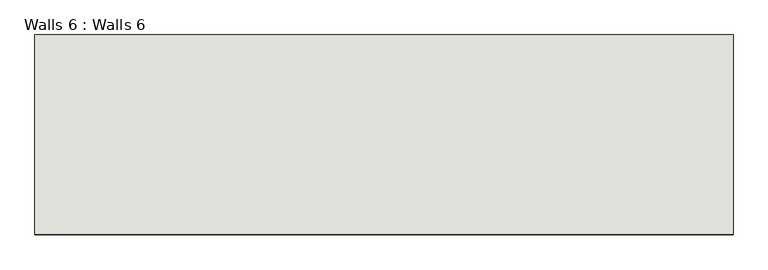
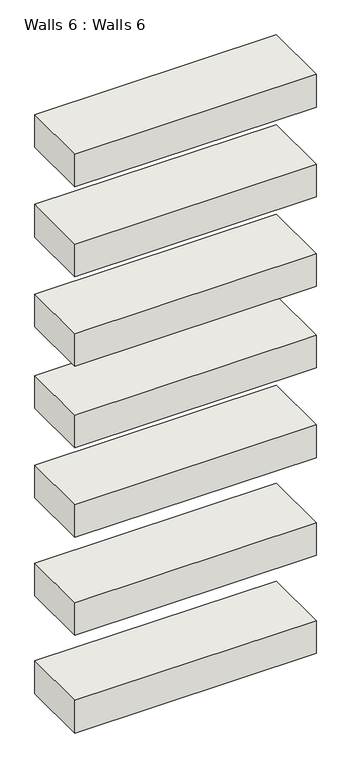
"""IFC4 building model written with IfcOpenShell, lengths in millimetres: wall geometry, Walls 6 : Walls 6."""

from ifc_helpers import new_model, si_unit, frame, origin, place, context, project, spatial, polyline, outline, extrude, source, transform, mapped, element, save


def walls_6_walls_6_ffd2a55d(model_context):
    return source(origin(), model_context, "Body", "SweptSolid", [
        extrude(outline(polyline([(-2720.1036351, 1505.9827135), (-3786.9036351, 1505.9827135), (-3786.9036351, 1810.7827135), (-2720.1036351, 1810.7827135), (-2720.1036351, 1505.9827135)])), frame((0.0, 0.0, 4076.7), z_axis=(0.0, 0.0, 1.0), x_axis=(1.0, 0.0, 0.0)), (0.0, 0.0, 1.0), 152.4),
        extrude(outline(polyline([(-2720.1036351, 1505.9827135), (-3786.9036351, 1505.9827135), (-3786.9036351, 1810.7827135), (-2720.1036351, 1810.7827135), (-2720.1036351, 1505.9827135)])), frame((0.0, 0.0, 3657.6), z_axis=(0.0, 0.0, 1.0), x_axis=(1.0, 0.0, 0.0)), (0.0, 0.0, 1.0), 152.4),
        extrude(outline(polyline([(-2720.1036351, 1505.9827135), (-3786.9036351, 1505.9827135), (-3786.9036351, 1810.7827135), (-2720.1036351, 1810.7827135), (-2720.1036351, 1505.9827135)])), frame((0.0, 0.0, 3238.5), z_axis=(0.0, 0.0, 1.0), x_axis=(1.0, 0.0, 0.0)), (0.0, 0.0, 1.0), 152.4),
        extrude(outline(polyline([(-2720.1036351, 1505.9827135), (-3786.9036351, 1505.9827135), (-3786.9036351, 1810.7827135), (-2720.1036351, 1810.7827135), (-2720.1036351, 1505.9827135)])), frame((0.0, 0.0, 2857.5), z_axis=(0.0, 0.0, 1.0), x_axis=(1.0, 0.0, 0.0)), (0.0, 0.0, 1.0), 152.4),
        extrude(outline(polyline([(-2720.1036351, 1505.9827135), (-3786.9036351, 1505.9827135), (-3786.9036351, 1810.7827135), (-2720.1036351, 1810.7827135), (-2720.1036351, 1505.9827135)])), frame((0.0, 0.0, 2438.4), z_axis=(0.0, 0.0, 1.0), x_axis=(1.0, 0.0, 0.0)), (0.0, 0.0, 1.0), 152.4),
        extrude(outline(polyline([(-2720.1036351, 1505.9827135), (-3786.9036351, 1505.9827135), (-3786.9036351, 1810.7827135), (-2720.1036351, 1810.7827135), (-2720.1036351, 1505.9827135)])), frame((0.0, 0.0, 1981.2), z_axis=(0.0, 0.0, 1.0), x_axis=(1.0, 0.0, 0.0)), (0.0, 0.0, 1.0), 152.4),
        extrude(outline(polyline([(-2720.1036351, 1505.9827135), (-3786.9036351, 1505.9827135), (-3786.9036351, 1810.7827135), (-2720.1036351, 1810.7827135), (-2720.1036351, 1505.9827135)])), frame((0.0, 0.0, 1524.0), z_axis=(0.0, 0.0, 1.0), x_axis=(1.0, 0.0, 0.0)), (0.0, 0.0, 1.0), 152.4),
    ])


if __name__ == "__main__":
    model = new_model("IFC4")
    model_context = context("Model", 3, world=origin())
    ifc_project = project(units=[si_unit("LENGTHUNIT", "METRE", prefix="MILLI")], contexts=[model_context])
    site = spatial("IfcSite", under=ifc_project)
    building = spatial("IfcBuilding", under=site)
    placement = place(None, origin())
    walls_6_walls_6_shape = walls_6_walls_6_ffd2a55d(model_context)
    element("IfcWall", 1, ObjectType="Walls 6 : Walls 6", at=placement, inside=building, context=model_context, shape_type="MappedRepresentation", body=[
        mapped(walls_6_walls_6_shape, transform((0.0, 0.0, 0.0), x_axis=(1.0, 0.0, 0.0), y_axis=(0.0, 1.0, 0.0), z_axis=(0.0, 0.0, 1.0))),
    ])
    save(model, "model.ifc")

# Revit data of these elements
# Element 1 (IfcWall, "Walls 6 : Walls 6")
#   Materials on its faces: "Default Wall"
# Materials
#   "Default Wall": colour RGB 128 128 128, transparency 0
